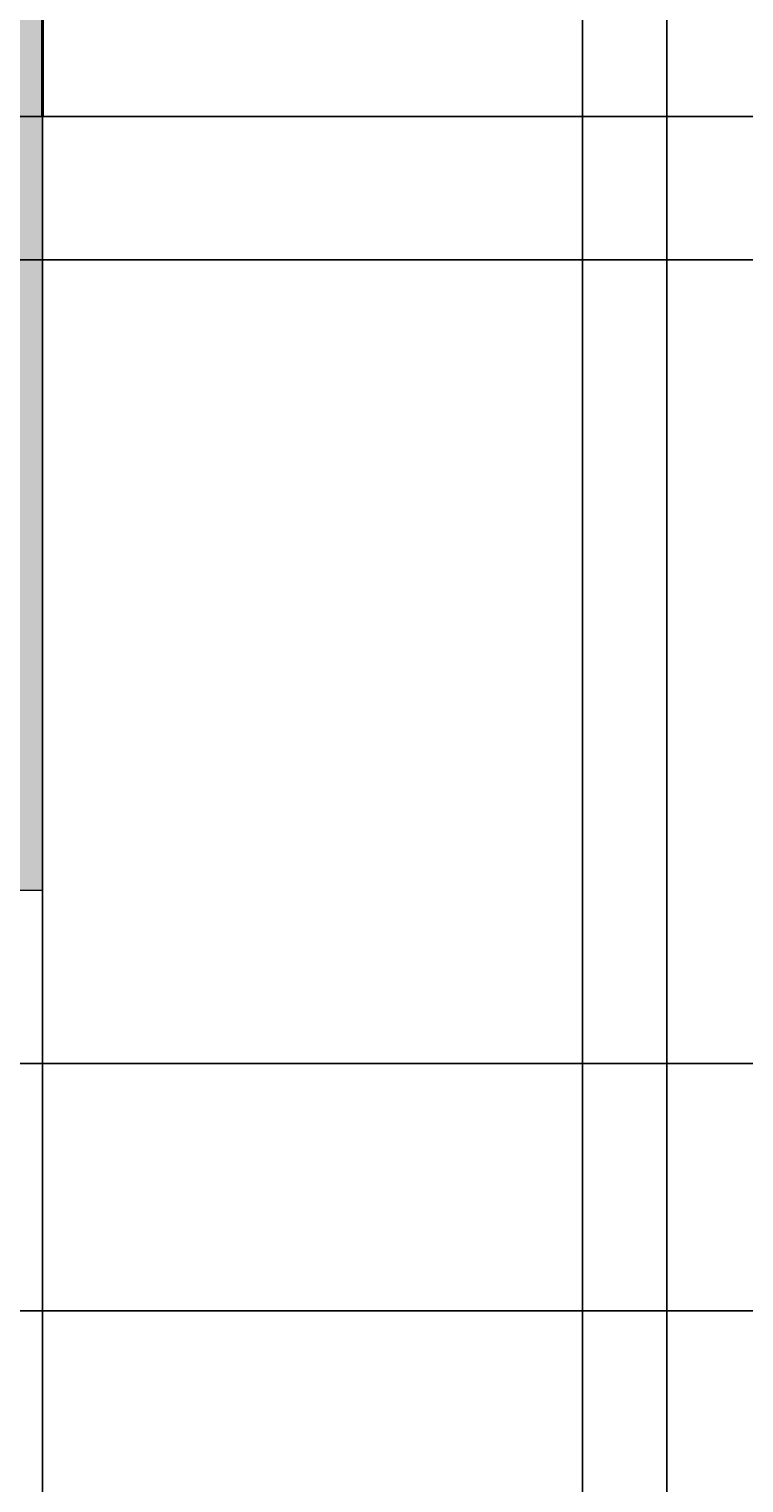
# Model space of a CAD drawing. Units: inches. Extents: x 818 to 1898, y 976 to 2364.
# Tile 41 of 96: x 1714 to 1750, y 1277 to 1350. Entities that reach past the tile are written whole.
import ezdxf

# ---------------------------------------------------------------- set-up
doc = ezdxf.new("R2010")
doc.units = ezdxf.units.IN
doc.header["$LTSCALE"] = 5
doc.header["$MEASUREMENT"] = 0
for name, color, linetype, lineweight in [('A-ANNO-DIMS', 2, 'Continuous', 18), ('A-WALL', 7, 'Continuous', 40), ('L-PLNT-BEDS', 94, 'Continuous', 18)]:
    doc.layers.add(name, color=color, linetype=linetype, lineweight=lineweight)
doc.layers.add('A-WALL-PATT', color=251, linetype='Continuous', lineweight=13, true_color=0x636466)
doc.styles.get("Standard").update_dxf_attribs({"font": 'arial.ttf'})
doc.dimstyles.get("Standard").update_dxf_attribs({"dimtxt": 0.18, "dimasz": 0.18, "dimexe": 0.18, "dimexo": 0.0625, "dimgap": 0.09, "dimtad": 0, "dimtih": 1, "dimtoh": 1, "dimdec": 4, "dimzin": 0, "dimdsep": 46, "dimtxsty": 'Standard', "dimcen": 0.09, "dimadec": 0, "dimazin": 0, "dimtfac": 1, "dimtdec": 4, "dimtofl": 0, "dimtmove": 0, "dimatfit": 3, "dimfxl": 1, "dimtolj": 1, "dimtzin": 0, "dimarcsym": 0})

# ---------------------------------------------------------------- blocks, each defined once
blk = doc.blocks.new('*D65')
at = {"layer": 'A-ANNO-DIMS', "color": 0, "lineweight": -2, "ltscale": 5, "transparency": 16777216}
for p, q in [((1430.725, 1346.016), (1430.725, 975.663)), ((1714.725, 1346.016), (1714.725, 975.663)), ((1430.905, 975.843), (1572.435, 975.843)), ((1714.545, 975.843), (1573.015, 975.843))]:
    blk.add_line(p, q, dxfattribs=at)
at = {"layer": 'A-ANNO-DIMS', "color": 0, "ltscale": 5, "transparency": 16777216}
for points in [[(1430.905, 975.873), (1430.905, 975.813), (1430.725, 975.843)], [(1714.545, 975.873), (1714.545, 975.813), (1714.725, 975.843)]]:
    blk.add_solid(points, dxfattribs=at)
at = {"layer": 'Defpoints', "color": 0, "ltscale": 5, "transparency": 16777216}
for p in [(1430.725, 1346.078), (1714.725, 1346.078), (1714.725, 975.843)]:
    blk.add_point(p, dxfattribs=at)
at = {"layer": 'A-ANNO-DIMS', "color": 0, "ltscale": 5, "transparency": 16777216, "insert": (1572.725, 975.843), "char_height": 0.18, "attachment_point": 5}
blk.add_mtext('\\A1;284', dxfattribs=at)
blk = doc.blocks.new('*D66')
at = {"layer": 'A-ANNO-DIMS', "color": 0, "lineweight": -2, "ltscale": 5, "transparency": 16777216}
for p, q in [((1714.725, 1346.016), (1714.725, 975.663)), ((1789.717, 1298.442), (1789.717, 975.663)), ((1714.905, 975.843), (1751.828, 975.843)), ((1789.537, 975.843), (1752.614, 975.843))]:
    blk.add_line(p, q, dxfattribs=at)
at = {"layer": 'A-ANNO-DIMS', "color": 0, "ltscale": 5, "transparency": 16777216}
for points in [[(1714.905, 975.873), (1714.905, 975.813), (1714.725, 975.843)], [(1789.537, 975.873), (1789.537, 975.813), (1789.717, 975.843)]]:
    blk.add_solid(points, dxfattribs=at)
at = {"layer": 'Defpoints', "color": 0, "ltscale": 5, "transparency": 16777216}
for p in [(1714.725, 1346.078), (1789.717, 1298.504), (1789.717, 975.843)]:
    blk.add_point(p, dxfattribs=at)
at = {"layer": 'A-ANNO-DIMS', "color": 0, "ltscale": 5, "transparency": 16777216, "insert": (1752.221, 975.843), "char_height": 0.18, "attachment_point": 5}
blk.add_mtext('\\A1;74.99', dxfattribs=at)
blk = doc.blocks.new('*D70')
at = {"layer": 'A-ANNO-DIMS', "color": 0, "lineweight": -2, "ltscale": 5, "transparency": 16777216}
for p, q in [((1714.788, 1346.078), (1897.916, 1346.078)), ((1897.736, 1345.898), (1897.736, 1274.703)), ((1897.736, 1203.144), (1897.736, 1274.339)), ((1798.78, 1202.964), (1897.916, 1202.964))]:
    blk.add_line(p, q, dxfattribs=at)
at = {"layer": 'A-ANNO-DIMS', "color": 0, "ltscale": 5, "transparency": 16777216}
for points in [[(1897.706, 1345.898), (1897.766, 1345.898), (1897.736, 1346.078)], [(1897.706, 1203.144), (1897.766, 1203.144), (1897.736, 1202.964)]]:
    blk.add_solid(points, dxfattribs=at)
at = {"layer": 'Defpoints', "color": 0, "ltscale": 5, "transparency": 16777216}
for p in [(1714.725, 1346.078), (1897.736, 1346.078), (1798.717, 1202.964)]:
    blk.add_point(p, dxfattribs=at)
at = {"layer": 'A-ANNO-DIMS', "color": 0, "ltscale": 5, "transparency": 16777216, "insert": (1897.736, 1274.521), "char_height": 0.18, "attachment_point": 5}
blk.add_mtext('\\A1;143.1', dxfattribs=at)
blk = doc.blocks.new('*D71')
at = {"layer": 'A-ANNO-DIMS', "color": 0, "lineweight": -2, "ltscale": 5, "transparency": 16777216}
for p, q in [((1714.788, 2053.078), (1897.916, 2053.078)), ((1897.736, 2052.898), (1897.736, 1699.76)), ((1897.736, 1346.258), (1897.736, 1699.396)), ((1714.788, 1346.078), (1897.916, 1346.078))]:
    blk.add_line(p, q, dxfattribs=at)
at = {"layer": 'A-ANNO-DIMS', "color": 0, "ltscale": 5, "transparency": 16777216}
for points in [[(1897.706, 2052.898), (1897.766, 2052.898), (1897.736, 2053.078)], [(1897.706, 1346.258), (1897.766, 1346.258), (1897.736, 1346.078)]]:
    blk.add_solid(points, dxfattribs=at)
at = {"layer": 'Defpoints', "color": 0, "ltscale": 5, "transparency": 16777216}
for p in [(1714.725, 2053.078), (1897.736, 2053.078), (1714.725, 1346.078)]:
    blk.add_point(p, dxfattribs=at)
at = {"layer": 'A-ANNO-DIMS', "color": 0, "ltscale": 5, "transparency": 16777216, "insert": (1897.736, 1699.578), "char_height": 0.18, "attachment_point": 5}
blk.add_mtext('\\A1;707', dxfattribs=at)
blk = doc.blocks.new('*D104')
at = {"layer": 'A-ANNO-DIMS', "color": 0, "lineweight": -2, "ltscale": 5, "transparency": 16777216}
for p, q in [((1689.471, 1071.118), (1689.471, 2363.873)), ((1689.651, 2363.693), (1717.401, 2363.693)), ((1745.903, 2363.693), (1718.154, 2363.693)), ((1746.083, 1071.118), (1746.083, 2363.873))]:
    blk.add_line(p, q, dxfattribs=at)
at = {"layer": 'A-ANNO-DIMS', "color": 0, "ltscale": 5, "transparency": 16777216}
for points in [[(1689.651, 2363.723), (1689.651, 2363.663), (1689.471, 2363.693)], [(1745.903, 2363.723), (1745.903, 2363.663), (1746.083, 2363.693)]]:
    blk.add_solid(points, dxfattribs=at)
at = {"layer": 'Defpoints', "color": 0, "ltscale": 5, "transparency": 16777216}
for p in [(1746.083, 2363.693), (1689.471, 1071.055), (1746.083, 1071.055)]:
    blk.add_point(p, dxfattribs=at)
at = {"layer": 'A-ANNO-DIMS', "color": 0, "ltscale": 5, "transparency": 16777216, "insert": (1717.777, 2363.693), "char_height": 0.18, "attachment_point": 5}
blk.add_mtext('\\A1;56.61', dxfattribs=at)
blk = doc.blocks.new('*D113')
at = {"layer": 'A-ANNO-DIMS', "color": 0, "lineweight": -2, "ltscale": 5, "transparency": 16777216}
for p, q in [((1430.788, 1346.078), (1897.916, 1346.078)), ((1897.736, 1345.898), (1897.736, 1316.26)), ((1897.736, 1286.258), (1897.736, 1315.896)), ((1430.788, 1286.078), (1897.916, 1286.078))]:
    blk.add_line(p, q, dxfattribs=at)
at = {"layer": 'A-ANNO-DIMS', "color": 0, "ltscale": 5, "transparency": 16777216}
for points in [[(1897.706, 1345.898), (1897.766, 1345.898), (1897.736, 1346.078)], [(1897.706, 1286.258), (1897.766, 1286.258), (1897.736, 1286.078)]]:
    blk.add_solid(points, dxfattribs=at)
at = {"layer": 'Defpoints', "color": 0, "ltscale": 5, "transparency": 16777216}
for p in [(1430.725, 1346.078), (1897.736, 1346.078), (1430.725, 1286.078)]:
    blk.add_point(p, dxfattribs=at)
at = {"layer": 'A-ANNO-DIMS', "color": 0, "ltscale": 5, "transparency": 16777216, "insert": (1897.736, 1316.078), "char_height": 0.18, "attachment_point": 5}
blk.add_mtext('\\A1;60', dxfattribs=at)
blk = doc.blocks.new('*D115')
at = {"layer": 'A-ANNO-DIMS', "color": 0, "lineweight": -2, "ltscale": 5, "transparency": 16777216}
for p, q in [((1766.29, 1377.656), (818.026, 1377.656)), ((818.206, 1377.476), (818.206, 1338.262)), ((818.206, 1298.684), (818.206, 1337.898)), ((1766.29, 1298.504), (818.026, 1298.504))]:
    blk.add_line(p, q, dxfattribs=at)
at = {"layer": 'A-ANNO-DIMS', "color": 0, "ltscale": 5, "transparency": 16777216}
for points in [[(818.176, 1377.476), (818.236, 1377.476), (818.206, 1377.656)], [(818.176, 1298.684), (818.236, 1298.684), (818.206, 1298.504)]]:
    blk.add_solid(points, dxfattribs=at)
at = {"layer": 'Defpoints', "color": 0, "ltscale": 5, "transparency": 16777216}
for p in [(818.206, 1377.656), (1766.352, 1377.656), (1766.352, 1298.504)]:
    blk.add_point(p, dxfattribs=at)
at = {"layer": 'A-ANNO-DIMS', "color": 0, "ltscale": 5, "transparency": 16777216, "insert": (818.206, 1338.08), "char_height": 0.18, "attachment_point": 5}
blk.add_mtext('\\A1;79.15', dxfattribs=at)
blk = doc.blocks.new('*D183')
at = {"layer": 'A-ANNO-DIMS', "color": 0, "lineweight": -2, "ltscale": 5, "transparency": 16777216}
for p, q in [((1714.725, 1545.016), (1714.725, 975.663)), ((1741.841, 1545.016), (1741.841, 975.663)), ((1714.905, 975.843), (1727.818, 975.843)), ((1741.661, 975.843), (1728.748, 975.843))]:
    blk.add_line(p, q, dxfattribs=at)
at = {"layer": 'A-ANNO-DIMS', "color": 0, "ltscale": 5, "transparency": 16777216}
for points in [[(1714.905, 975.873), (1714.905, 975.813), (1714.725, 975.843)], [(1741.661, 975.873), (1741.661, 975.813), (1741.841, 975.843)]]:
    blk.add_solid(points, dxfattribs=at)
at = {"layer": 'Defpoints', "color": 0, "ltscale": 5, "transparency": 16777216}
for p in [(1714.725, 1545.078), (1741.841, 1545.078), (1741.841, 975.843)]:
    blk.add_point(p, dxfattribs=at)
at = {"layer": 'A-ANNO-DIMS', "color": 0, "ltscale": 5, "transparency": 16777216, "insert": (1728.283, 975.843), "char_height": 0.18, "attachment_point": 5}
blk.add_mtext('\\A1;27.116', dxfattribs=at)
blk = doc.blocks.new('*D188')
at = {"layer": 'A-ANNO-DIMS', "color": 0, "lineweight": -2, "ltscale": 5, "transparency": 16777216}
for p, q in [((1714.788, 1545.078), (1897.916, 1545.078)), ((1897.736, 1544.898), (1897.736, 1445.76)), ((1897.736, 1346.258), (1897.736, 1445.396)), ((1714.788, 1346.078), (1897.916, 1346.078))]:
    blk.add_line(p, q, dxfattribs=at)
at = {"layer": 'A-ANNO-DIMS', "color": 0, "ltscale": 5, "transparency": 16777216}
for points in [[(1897.706, 1544.898), (1897.766, 1544.898), (1897.736, 1545.078)], [(1897.706, 1346.258), (1897.766, 1346.258), (1897.736, 1346.078)]]:
    blk.add_solid(points, dxfattribs=at)
at = {"layer": 'Defpoints', "color": 0, "ltscale": 5, "transparency": 16777216}
for p in [(1714.725, 1545.078), (1897.736, 1545.078), (1714.725, 1346.078)]:
    blk.add_point(p, dxfattribs=at)
at = {"layer": 'A-ANNO-DIMS', "color": 0, "ltscale": 5, "transparency": 16777216, "insert": (1897.736, 1445.578), "char_height": 0.18, "attachment_point": 5}
blk.add_mtext('\\A1;199', dxfattribs=at)
blk = doc.blocks.new('*D193')
at = {"layer": 'A-ANNO-DIMS', "color": 0, "lineweight": -2, "ltscale": 5, "transparency": 16777216}
for p, q in [((1660.377, 1346.078), (1897.916, 1346.078)), ((1897.736, 1345.898), (1897.736, 1342.654)), ((1897.736, 1339.045), (1897.736, 1342.29)), ((1660.377, 1338.865), (1897.916, 1338.865))]:
    blk.add_line(p, q, dxfattribs=at)
at = {"layer": 'A-ANNO-DIMS', "color": 0, "ltscale": 5, "transparency": 16777216}
for points in [[(1897.706, 1345.898), (1897.766, 1345.898), (1897.736, 1346.078)], [(1897.706, 1339.045), (1897.766, 1339.045), (1897.736, 1338.865)]]:
    blk.add_solid(points, dxfattribs=at)
at = {"layer": 'Defpoints', "color": 0, "ltscale": 5, "transparency": 16777216}
for p in [(1660.314, 1346.078), (1897.736, 1346.078), (1660.314, 1338.865)]:
    blk.add_point(p, dxfattribs=at)
at = {"layer": 'A-ANNO-DIMS', "color": 0, "ltscale": 5, "transparency": 16777216, "insert": (1897.736, 1342.472), "char_height": 0.18, "attachment_point": 5}
blk.add_mtext('\\A1;7.213', dxfattribs=at)
blk = doc.blocks.new('*D198')
at = {"layer": 'A-ANNO-DIMS', "color": 0, "lineweight": -2, "ltscale": 5, "transparency": 16777216}
for p, q in [((1741.841, 1545.016), (1741.841, 975.663)), ((1430.725, 1346.016), (1430.725, 975.663)), ((1430.905, 975.843), (1585.907, 975.843)), ((1741.661, 975.843), (1586.659, 975.843))]:
    blk.add_line(p, q, dxfattribs=at)
at = {"layer": 'A-ANNO-DIMS', "color": 0, "ltscale": 5, "transparency": 16777216}
for points in [[(1430.905, 975.873), (1430.905, 975.813), (1430.725, 975.843)], [(1741.661, 975.873), (1741.661, 975.813), (1741.841, 975.843)]]:
    blk.add_solid(points, dxfattribs=at)
at = {"layer": 'Defpoints', "color": 0, "ltscale": 5, "transparency": 16777216}
for p in [(1741.841, 1545.078), (1430.725, 1346.078), (1741.841, 975.843)]:
    blk.add_point(p, dxfattribs=at)
at = {"layer": 'A-ANNO-DIMS', "color": 0, "ltscale": 5, "transparency": 16777216, "insert": (1586.283, 975.843), "char_height": 0.18, "attachment_point": 5}
blk.add_mtext('\\A1;311.1', dxfattribs=at)
blk = doc.blocks.new('*D199')
at = {"layer": 'A-ANNO-DIMS', "color": 0, "lineweight": -2, "ltscale": 5, "transparency": 16777216}
for p, q in [((1559.788, 1687.078), (1897.916, 1687.078)), ((1897.736, 1686.898), (1897.736, 1513.154)), ((1897.736, 1339.045), (1897.736, 1512.79)), ((1660.377, 1338.865), (1897.916, 1338.865))]:
    blk.add_line(p, q, dxfattribs=at)
at = {"layer": 'A-ANNO-DIMS', "color": 0, "ltscale": 5, "transparency": 16777216}
for points in [[(1897.706, 1686.898), (1897.766, 1686.898), (1897.736, 1687.078)], [(1897.706, 1339.045), (1897.766, 1339.045), (1897.736, 1338.865)]]:
    blk.add_solid(points, dxfattribs=at)
at = {"layer": 'Defpoints', "color": 0, "ltscale": 5, "transparency": 16777216}
for p in [(1559.725, 1687.078), (1897.736, 1687.078), (1660.314, 1338.865)]:
    blk.add_point(p, dxfattribs=at)
at = {"layer": 'A-ANNO-DIMS', "color": 0, "ltscale": 5, "transparency": 16777216, "insert": (1897.736, 1512.972), "char_height": 0.18, "attachment_point": 5}
blk.add_mtext('\\A1;348.2', dxfattribs=at)
blk = doc.blocks.new('*D214')
at = {"layer": 'A-ANNO-DIMS', "color": 0, "lineweight": -2, "ltscale": 5, "transparency": 16777216}
for p, q in [((1511.725, 1687.016), (1511.725, 975.663)), ((1714.725, 1687.016), (1714.725, 975.663)), ((1511.905, 975.843), (1612.935, 975.843)), ((1714.545, 975.843), (1613.516, 975.843))]:
    blk.add_line(p, q, dxfattribs=at)
at = {"layer": 'A-ANNO-DIMS', "color": 0, "ltscale": 5, "transparency": 16777216}
for points in [[(1511.905, 975.873), (1511.905, 975.813), (1511.725, 975.843)], [(1714.545, 975.873), (1714.545, 975.813), (1714.725, 975.843)]]:
    blk.add_solid(points, dxfattribs=at)
at = {"layer": 'Defpoints', "color": 0, "ltscale": 5, "transparency": 16777216}
for p in [(1511.725, 1687.078), (1714.725, 1687.078), (1714.725, 975.843)]:
    blk.add_point(p, dxfattribs=at)
at = {"layer": 'A-ANNO-DIMS', "color": 0, "ltscale": 5, "transparency": 16777216, "insert": (1613.225, 975.843), "char_height": 0.18, "attachment_point": 5}
blk.add_mtext('\\A1;203', dxfattribs=at)
blk = doc.blocks.new('*D267')
at = {"layer": 'A-ANNO-DIMS', "color": 0, "lineweight": -2, "ltscale": 5, "transparency": 16777216}
for p, q in [((1714.725, 1687.016), (1714.725, 975.663)), ((1741.841, 1687.016), (1741.841, 975.663)), ((1714.905, 975.843), (1727.818, 975.843)), ((1741.661, 975.843), (1728.748, 975.843))]:
    blk.add_line(p, q, dxfattribs=at)
at = {"layer": 'A-ANNO-DIMS', "color": 0, "ltscale": 5, "transparency": 16777216}
for points in [[(1714.905, 975.873), (1714.905, 975.813), (1714.725, 975.843)], [(1741.661, 975.873), (1741.661, 975.813), (1741.841, 975.843)]]:
    blk.add_solid(points, dxfattribs=at)
at = {"layer": 'Defpoints', "color": 0, "ltscale": 5, "transparency": 16777216}
for p in [(1714.725, 1687.078), (1741.841, 1687.078), (1741.841, 975.843)]:
    blk.add_point(p, dxfattribs=at)
at = {"layer": 'A-ANNO-DIMS', "color": 0, "ltscale": 5, "transparency": 16777216, "insert": (1728.283, 975.843), "char_height": 0.18, "attachment_point": 5}
blk.add_mtext('\\A1;27.116', dxfattribs=at)

msp = doc.modelspace()

# ---------------------------------------------------------------- hatches: boundary and pattern name
at = {"layer": 'A-WALL-PATT', "ltscale": 5}
h = msp.add_hatch(color=256, dxfattribs=at)
h.dxf.hatch_style = 1
h.paths.add_polyline_path([(1714.7251, 1521.0782), (1705.7252, 1521.0782), (1705.7252, 1467.0782), (1654.7252, 1467.0782), (1654.7252, 1463.0782), (1705.7252, 1463.0782), (1705.7252, 1355.0782), (1622.7252, 1355.0782), (1622.7252, 1379.0782), (1622.7252, 1386.6857), (1616.7252, 1386.6857), (1616.7252, 1355.0782), (1490.9163, 1355.0782), (1490.9163, 1346.0782), (1544.7605, 1346.0782), (1544.6132, 1346.8783), (1544.6729, 1346.84), (1544.6299, 1346.7874), (1544.7605, 1346.0782), (1555.1299, 1346.0782), (1555.1299, 1341.5528), (1556.1599, 1340.8639), (1556.5281, 1338.8654), (1660.3141, 1338.8654), (1660.3141, 1346.0782), (1705.7252, 1346.0782), (1705.7252, 1345.0768), (1705.8704, 1344.58), (1705.7252, 1344.3933), (1705.7252, 1334.9904), (1705.8704, 1334.4936), (1705.7252, 1334.3068), (1705.7252, 1316.2253), (1707.3573, 1316.7694), (1707.3847, 1316.8046), (1707.3807, 1316.7771), (1705.7252, 1316.2253), (1705.7252, 1314.1392), (1705.7252, 1312.0957), (1705.8703, 1312.0739), (1705.7252, 1311.8873), (1705.7252, 1310.7121), (1706.5603, 1307.9282), (1707.8887, 1307.1831), (1714.7251, 1307.1831), (1714.7251, 1346.0782)])

# ---------------------------------------------------------------- linework, layer by layer
at = {"layer": 'A-WALL'}
msp.add_line((1714.7251, 1545.0782), (1714.7251, 1346.0782), dxfattribs=at)
at = {"layer": 'L-PLNT-BEDS', "ltscale": 5}
for p, q in [((1714.7251, 1346.0782), (1714.7251, 1307.1831)), ((1714.7251, 1307.1831), (1705.7252, 1307.1831))]:
    msp.add_line(p, q, dxfattribs=at)

# ---------------------------------------------------------------- dimensions: what is measured, and where the dimension line sits
at = {"layer": 'A-ANNO-DIMS', "ltscale": 5}
for base, p1, p2, override, picture, middle in [((1746.0831, 2363.6929), (1689.4714, 1071.0552), (1746.0831, 1071.0552), {"dimdec": 2, "dimlfac": 1, "dimrnd": 0, "dimzin": 0, "dimdsep": 46, "dimlunit": 2}, '*D104', (1717.7772, 2363.6929)), ((1714.7251, 975.8433), (1511.7251, 1687.0782), (1714.7251, 1687.0782), {"dimdec": 0, "dimlfac": 1, "dimrnd": 0, "dimzin": 0, "dimdsep": 46, "dimlunit": 2}, '*D214', (1613.2251, 975.8433)), ((1741.8409, 975.8433), (1714.7251, 1687.0782), (1741.8409, 1687.0782), {"dimdec": 3, "dimlfac": 1, "dimrnd": 0, "dimzin": 0, "dimdsep": 46, "dimlunit": 2}, '*D267', (1728.283, 975.8433)), ((1741.8409, 975.8433), (1430.7251, 1346.0782), (1741.8409, 1545.0782), {"dimdec": 1, "dimlfac": 1, "dimrnd": 0, "dimzin": 0, "dimdsep": 46, "dimlunit": 2}, '*D198', (1586.283, 975.8433)), ((1741.8409, 975.8433), (1714.7251, 1545.0782), (1741.8409, 1545.0782), {"dimdec": 3, "dimlfac": 1, "dimrnd": 0, "dimzin": 0, "dimdsep": 46, "dimlunit": 2}, '*D183', (1728.283, 975.8433)), ((1714.7251, 975.8433), (1430.7251, 1346.0782), (1714.7251, 1346.0782), {"dimdec": 0, "dimlfac": 1, "dimrnd": 0, "dimzin": 0, "dimdsep": 46, "dimlunit": 2}, '*D65', (1572.7251, 975.8433)), ((1789.7173, 975.8433), (1714.7251, 1346.0782), (1789.7173, 1298.5041), {"dimdec": 2, "dimlfac": 1, "dimrnd": 0, "dimzin": 0, "dimdsep": 46, "dimlunit": 2}, '*D66', (1752.2212, 975.8433))]:
    dim = msp.add_linear_dim(base=base, p1=p1, p2=p2, dimstyle='Standard', override=override, dxfattribs=at)
    dim.commit()
    dim.dimension.update_dxf_attribs({"geometry": picture, "text_midpoint": middle})
for base, p1, p2, override, picture, middle in [((1897.736, 2053.0782), (1714.7251, 1346.0782), (1714.7251, 2053.0782), {"dimdec": 0, "dimlfac": 1, "dimrnd": 0, "dimzin": 0, "dimdsep": 46, "dimlunit": 2}, '*D71', (1897.736, 1699.5782)), ((1897.736, 1687.0782), (1660.3141, 1338.8654), (1559.7251, 1687.0782), {"dimdec": 1, "dimlfac": 1, "dimrnd": 0, "dimzin": 0, "dimdsep": 46, "dimlunit": 2}, '*D199', (1897.736, 1512.9718)), ((1897.736, 1545.0782), (1714.7251, 1346.0782), (1714.7251, 1545.0782), {"dimdec": 0, "dimlfac": 1, "dimrnd": 0, "dimzin": 0, "dimdsep": 46, "dimlunit": 2}, '*D188', (1897.736, 1445.5782)), ((818.2059, 1377.6564), (1766.3524, 1298.5041), (1766.3524, 1377.6564), {"dimdec": 2, "dimlfac": 1, "dimrnd": 0, "dimzin": 0, "dimdsep": 46, "dimlunit": 2}, '*D115', (818.2059, 1338.0803)), ((1897.736, 1346.0782), (1430.7251, 1286.0782), (1430.7251, 1346.0782), {"dimdec": 0, "dimlfac": 1, "dimrnd": 0, "dimzin": 0, "dimdsep": 46, "dimlunit": 2}, '*D113', (1897.736, 1316.0782)), ((1897.736, 1346.0782), (1660.3141, 1338.8654), (1660.3141, 1346.0782), {"dimdec": 3, "dimlfac": 1, "dimrnd": 0, "dimzin": 0, "dimdsep": 46, "dimlunit": 2}, '*D193', (1897.736, 1342.4718)), ((1897.736, 1346.0782), (1798.7173, 1202.9642), (1714.7251, 1346.0782), {"dimdec": 1, "dimlfac": 1, "dimrnd": 0, "dimzin": 0, "dimdsep": 46, "dimlunit": 2}, '*D70', (1897.736, 1274.5212))]:
    dim = msp.add_linear_dim(base=base, p1=p1, p2=p2, angle=90, dimstyle='Standard', override=override, dxfattribs=at)
    dim.commit()
    dim.dimension.update_dxf_attribs({"geometry": picture, "text_midpoint": middle})

doc.saveas('drawing.dxf')
